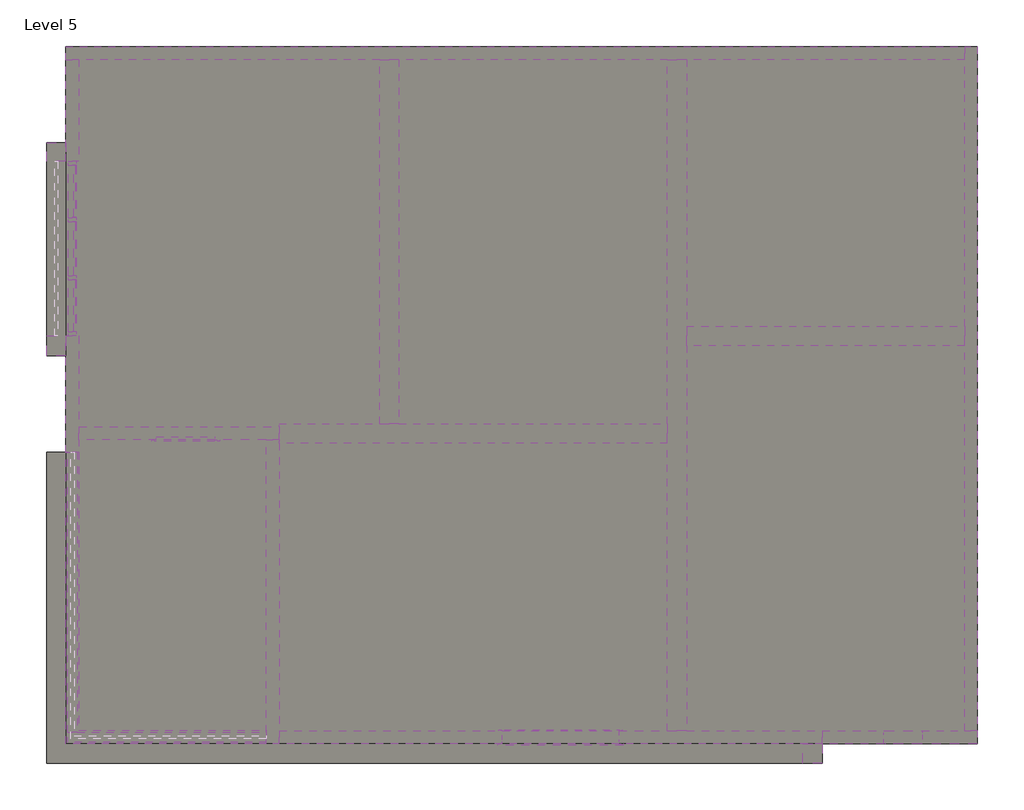
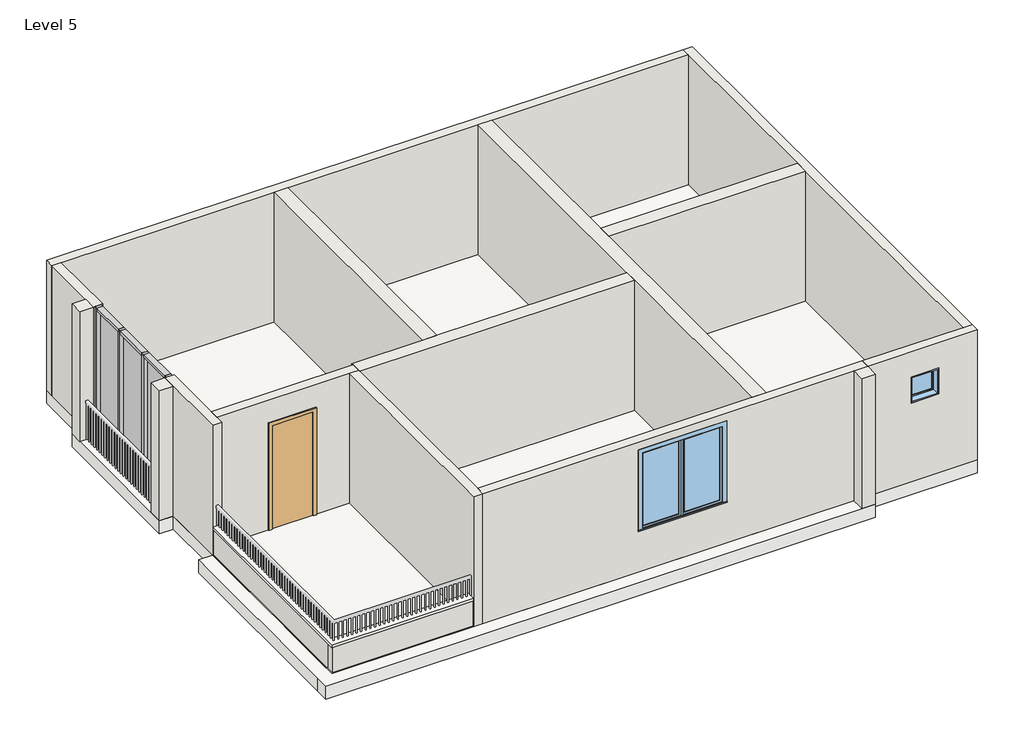
# One storey, part 1 of 2: 17 walls, 10 members, 3 plates, 3 slabs, 2 windows, 1 door.
"""IFC4 building model written with IfcOpenShell, lengths in millimetres."""

from ifc_helpers import new_model, si_unit, frame, origin, place, context, project, spatial, polyline, outline, extrude, faceted_brep, transform, mapped, element, save
from components import door_f936a269, member_eaba9652, member_3f395ae9, member_c17f1be2, member_d2e7e466, system_panel_glazed_52d31088, system_panel_glazed_f0722de2, window_97c6202a, window_6846e476

model = new_model("IFC4")

# Units and contexts
model_context = context("Model", 3, world=origin())
ifc_project = project(units=[si_unit("LENGTHUNIT", "METRE", prefix="MILLI")], contexts=[model_context])

# Site, building, storey
site = spatial("IfcSite", under=ifc_project)
building = spatial("IfcBuilding", under=site)
storey = spatial("IfcBuildingStorey", under=building, Name="Level 5", Elevation=12192.0)

# Door
placement = place(None, origin())
door_shape = door_f936a269(model_context)
element("IfcDoor", 1, ObjectType="Single-Flush : 36\" x 96\"", at=placement, inside=storey, context=model_context, shape_type="MappedRepresentation", body=[
    mapped(door_shape, transform((-16449.2169582, -4610.4617616, 13411.2), x_axis=(-1.0, 0.0, 0.0), y_axis=(0.0, -1.0, 0.0), z_axis=(0.0, 0.0, 1.0))),
])

# Members
member_shape = member_eaba9652(model_context)
element("IfcMember", 2, ObjectType="Rectangular Mullion : 2.5\" x 5\" rectangular", at=placement, inside=storey, context=model_context, shape_type="MappedRepresentation", body=[
    mapped(member_shape, transform((-18227.2169582, -1251.3117616, 13411.2), x_axis=(0.0, -1.0, 0.0), y_axis=(-1.0, 0.0, 0.0), z_axis=(0.0, 0.0, -1.0))),
])
element("IfcMember", 3, ObjectType="Rectangular Mullion : 2.5\" x 5\" rectangular", at=placement, inside=storey, context=model_context, shape_type="MappedRepresentation", body=[
    mapped(member_shape, transform((-18227.2169582, -2165.7117616, 13411.2), x_axis=(0.0, -1.0, 0.0), y_axis=(-1.0, 0.0, 0.0), z_axis=(0.0, 0.0, -1.0))),
])
member_2_shape = member_3f395ae9(model_context)
element("IfcMember", 4, ObjectType="Rectangular Mullion : 2.5\" x 5\" rectangular", at=placement, inside=storey, context=model_context, shape_type="MappedRepresentation", body=[
    mapped(member_2_shape, transform((-18227.2169582, -3080.1117616, 13411.2), x_axis=(0.0, -1.0, 0.0), y_axis=(-1.0, 0.0, 0.0), z_axis=(0.0, 0.0, -1.0))),
])
element("IfcMember", 5, ObjectType="Rectangular Mullion : 2.5\" x 5\" rectangular", at=placement, inside=storey, context=model_context, shape_type="MappedRepresentation", body=[
    mapped(member_2_shape, transform((-18227.2169582, -336.9117616, 16459.2), x_axis=(0.0, 1.0, 0.0), y_axis=(-1.0, 0.0, 0.0), z_axis=(0.0, 0.0, 1.0))),
])
member_3_shape = member_c17f1be2(model_context)
element("IfcMember", 6, ObjectType="Rectangular Mullion : 2.5\" x 5\" rectangular", at=placement, inside=storey, context=model_context, shape_type="MappedRepresentation", body=[
    mapped(member_3_shape, transform((-18227.2169582, -3016.6117616, 16459.2), x_axis=(0.0, 0.0, 1.0), y_axis=(-1.0, 0.0, 0.0), z_axis=(0.0, -1.0, 0.0))),
])
element("IfcMember", 7, ObjectType="Rectangular Mullion : 2.5\" x 5\" rectangular", at=placement, inside=storey, context=model_context, shape_type="MappedRepresentation", body=[
    mapped(member_3_shape, transform((-18227.2169582, -1219.5617616, 16459.2), x_axis=(0.0, 0.0, 1.0), y_axis=(-1.0, 0.0, 0.0), z_axis=(0.0, -1.0, 0.0))),
])
element("IfcMember", 8, ObjectType="Rectangular Mullion : 2.5\" x 5\" rectangular", at=placement, inside=storey, context=model_context, shape_type="MappedRepresentation", body=[
    mapped(member_3_shape, transform((-18227.2169582, -400.4117616, 13411.2), x_axis=(0.0, 0.0, -1.0), y_axis=(-1.0, 0.0, 0.0), z_axis=(0.0, 1.0, 0.0))),
])
element("IfcMember", 9, ObjectType="Rectangular Mullion : 2.5\" x 5\" rectangular", at=placement, inside=storey, context=model_context, shape_type="MappedRepresentation", body=[
    mapped(member_3_shape, transform((-18227.2169582, -2197.4617616, 13411.2), x_axis=(0.0, 0.0, -1.0), y_axis=(-1.0, 0.0, 0.0), z_axis=(0.0, 1.0, 0.0))),
])
member_4_shape = member_d2e7e466(model_context)
element("IfcMember", 10, ObjectType="Rectangular Mullion : 2.5\" x 5\" rectangular", at=placement, inside=storey, context=model_context, shape_type="MappedRepresentation", body=[
    mapped(member_4_shape, transform((-18227.2169582, -1283.0617616, 13411.2), x_axis=(0.0, 0.0, -1.0), y_axis=(-1.0, 0.0, 0.0), z_axis=(0.0, 1.0, 0.0))),
])
element("IfcMember", 11, ObjectType="Rectangular Mullion : 2.5\" x 5\" rectangular", at=placement, inside=storey, context=model_context, shape_type="MappedRepresentation", body=[
    mapped(member_4_shape, transform((-18227.2169582, -2133.9617616, 16459.2), x_axis=(0.0, 0.0, 1.0), y_axis=(-1.0, 0.0, 0.0), z_axis=(0.0, -1.0, 0.0))),
])

# Plates
system_panel_glazed_shape = system_panel_glazed_52d31088(model_context)
element("IfcPlate", 12, ObjectType="System Panel : Glazed", at=placement, inside=storey, context=model_context, shape_type="MappedRepresentation", body=[
    mapped(system_panel_glazed_shape, transform((-18227.2169582, -809.9867616, 13474.7), x_axis=(0.0, -1.0, 0.0), y_axis=(1.0, 0.0, 0.0), z_axis=(0.0, 0.0, 1.0))),
])
element("IfcPlate", 13, ObjectType="System Panel : Glazed", at=placement, inside=storey, context=model_context, shape_type="MappedRepresentation", body=[
    mapped(system_panel_glazed_shape, transform((-18227.2169582, -2607.0367616, 13474.7), x_axis=(0.0, -1.0, 0.0), y_axis=(1.0, 0.0, 0.0), z_axis=(0.0, 0.0, 1.0))),
])
system_panel_glazed_2_shape = system_panel_glazed_f0722de2(model_context)
element("IfcPlate", 14, ObjectType="System Panel : Glazed", at=placement, inside=storey, context=model_context, shape_type="MappedRepresentation", body=[
    mapped(system_panel_glazed_2_shape, transform((-18227.2169582, -1708.5117616, 13474.7), x_axis=(0.0, -1.0, 0.0), y_axis=(1.0, 0.0, 0.0), z_axis=(0.0, 0.0, 1.0))),
])

# Slabs
element("IfcSlab", 15, ObjectType="Generic - 12\"", at=placement, inside=storey, context=model_context, shape_type="SweptSolid", body=[
    extrude(outline(polyline([(-18633.6169582, -41.6299243), (-18328.8169582, -41.6299243), (-18328.8169582, -3394.4299243), (-18633.6169582, -3394.4299243), (-18633.6169582, -41.6299243)])), frame((0.0, 0.0, 13106.4), z_axis=(0.0, 0.0, 1.0), x_axis=(1.0, 0.0, 0.0)), (0.0, 0.0, 1.0), 304.8),
    extrude(outline(polyline([(-18633.6169582, -4908.9117616), (-18328.8169582, -4908.9117616), (-18328.8169582, -9487.2617616), (-6444.7919582, -9487.2617616), (-6444.7919582, -9792.0617616), (-18633.6169582, -9792.0617616), (-18633.6169582, -9487.2617616), (-18633.6169582, -4908.9117616)])), frame((0.0, 0.0, 13106.4), z_axis=(0.0, 0.0, 1.0), x_axis=(1.0, 0.0, 0.0)), (0.0, 0.0, 1.0), 304.8),
])
element("IfcSlab", 16, ObjectType="Generic - 12\" 2", at=placement, inside=storey, context=model_context, shape_type="SweptSolid", body=[
    extrude(outline(polyline([(-4006.3919582, 1466.4882384), (-4006.3919582, -9487.2617616), (-18328.8169582, -9487.2617616), (-18328.8169582, 1466.4882384), (-4006.3919582, 1466.4882384)])), frame((0.0, 0.0, 13106.4), z_axis=(0.0, 0.0, 1.0), x_axis=(1.0, 0.0, 0.0)), (0.0, 0.0, 1.0), 304.8),
])
element("IfcSlab", 17, ObjectType="Generic - 2\"", at=placement, inside=storey, context=model_context, shape_type="SweptSolid", body=[
    extrude(outline(polyline([(-15179.2169582, -9487.2617616), (-18328.8169582, -9487.2617616), (-18328.8169582, -4908.9117616), (-18125.6169582, -4908.9117616), (-18125.6169582, -9277.7117616), (-15179.2169582, -9277.7117616), (-15179.2169582, -9309.4617616), (-15179.2169582, -9487.2617616)])), frame((0.0, 0.0, 14020.8), z_axis=(0.0, 0.0, 1.0), x_axis=(1.0, 0.0, 0.0)), (0.0, 0.0, 1.0), 50.8),
])

# Walls
element("IfcWall", 18, ObjectType="Generic - 12\" white", at=placement, inside=storey, context=model_context, shape_type="SweptSolid", body=[
    extrude(outline(polyline([(-18633.6169582, -336.9117616), (-18633.6169582, -41.6299243), (-18328.8169582, -41.6299243), (-18328.8169582, -336.9117616), (-18633.6169582, -336.9117616)])), frame((0.0, 0.0, 13411.2), z_axis=(0.0, 0.0, 1.0), x_axis=(1.0, 0.0, 0.0)), (0.0, 0.0, 1.0), 3048.0),
])
element("IfcWall", 19, ObjectType="Generic - 12\" white", at=placement, inside=storey, context=model_context, shape_type="SweptSolid", body=[
    extrude(outline(polyline([(-18328.8169582, -3080.1117616), (-18328.8169582, -3394.4299243), (-18633.6169582, -3394.4299243), (-18633.6169582, -3080.1117616), (-18328.8169582, -3080.1117616)])), frame((0.0, 0.0, 13411.2), z_axis=(0.0, 0.0, 1.0), x_axis=(1.0, 0.0, 0.0)), (0.0, 0.0, 1.0), 3048.0),
])
element("IfcWall", 20, ObjectType="Generic - 12\" white", at=placement, inside=storey, context=model_context, shape_type="SweptSolid", body=[
    extrude(outline(polyline([(-6749.5919582, -9487.2617616), (-6444.7919582, -9487.2617616), (-6444.7919582, -9792.0617616), (-6749.5919582, -9792.0617616), (-6749.5919582, -9487.2617616)])), frame((0.0, 0.0, 13411.2), z_axis=(0.0, 0.0, 1.0), x_axis=(1.0, 0.0, 0.0)), (0.0, 0.0, 1.0), 3048.0),
])
element("IfcWall", 21, ObjectType="Generic - 12\" white", at=placement, inside=storey, context=model_context, shape_type="Brep", body=[
    faceted_brep([(-8575.2169582, -9284.0617616, 13411.2), (-8575.2169582, -3232.5117616, 13411.2), (-8575.2169582, -2927.7117616, 13411.2), (-8575.2169582, 1263.2882384, 13411.2), (-8575.2169582, 1263.2882384, 16459.2), (-8575.2169582, -2927.7117616, 16459.2), (-8575.2169582, -3232.5117616, 16459.2), (-8575.2169582, -9284.0617616, 16459.2), (-8880.0169582, -9284.0617616, 13411.2), (-8880.0169582, -9284.0617616, 16459.2), (-8880.0169582, -4762.8617616, 16459.2), (-8880.0169582, -4458.0617616, 16459.2), (-8880.0169582, 1263.2882384, 16459.2), (-8880.0169582, 1263.2882384, 13411.2), (-8880.0169582, -4458.0617616, 13411.2), (-8880.0169582, -4762.8617616, 13411.2)], [[[0, 1, 2, 3, 4, 5, 6, 7]], [[8, 9, 10, 11, 12, 13, 14, 15]], [[3, 2, 1, 0, 8, 15, 14, 13]], [[7, 6, 5, 4, 12, 11, 10, 9]], [[4, 3, 13, 12]], [[0, 7, 9, 8]]]),
])
element("IfcWall", 22, ObjectType="Generic - 12\" white", at=placement, inside=storey, context=model_context, shape_type="Brep", body=[
    faceted_brep([(-14976.0169582, -4762.8617616, 13411.2), (-8880.0169582, -4762.8617616, 13411.2), (-8880.0169582, -4762.8617616, 16459.2), (-14976.0169582, -4762.8617616, 16459.2), (-14976.0169582, -4458.0617616, 13411.2), (-14976.0169582, -4458.0617616, 16459.2), (-13401.2169582, -4458.0617616, 16459.2), (-13096.4169582, -4458.0617616, 16459.2), (-8880.0169582, -4458.0617616, 16459.2), (-8880.0169582, -4458.0617616, 13411.2), (-13096.4169582, -4458.0617616, 13411.2), (-13401.2169582, -4458.0617616, 13411.2), (-14976.0169582, -4712.0617616, 13411.2), (-14976.0169582, -4508.8617616, 13411.2), (-14976.0169582, -4508.8617616, 16459.2), (-14976.0169582, -4712.0617616, 16459.2)], [[[0, 1, 2, 3]], [[4, 5, 6, 7, 8, 9, 10, 11]], [[1, 0, 12, 13, 4, 11, 10, 9]], [[3, 2, 8, 7, 6, 5, 14, 15]], [[0, 3, 15, 14, 5, 4, 13, 12]], [[2, 1, 9, 8]]]),
])
element("IfcWall", 23, ObjectType="Generic - 12\" white", at=placement, inside=storey, context=model_context, shape_type="SweptSolid", body=[
    extrude(outline(polyline([(-13096.4169582, 1263.2882384), (-13096.4169582, -4458.0617616), (-13401.2169582, -4458.0617616), (-13401.2169582, 1263.2882384), (-13096.4169582, 1263.2882384)])), frame((0.0, 0.0, 13411.2), z_axis=(0.0, 0.0, 1.0), x_axis=(1.0, 0.0, 0.0)), (0.0, 0.0, 1.0), 3048.0),
])
element("IfcWall", 24, ObjectType="Generic - 12\" white", at=placement, inside=storey, context=model_context, shape_type="SweptSolid", body=[
    extrude(outline(polyline([(-4209.5919582, -3232.5117616), (-8575.2169582, -3232.5117616), (-8575.2169582, -2927.7117616), (-4209.5919582, -2927.7117616), (-4209.5919582, -3232.5117616)])), frame((0.0, 0.0, 13411.2), z_axis=(0.0, 0.0, 1.0), x_axis=(1.0, 0.0, 0.0)), (0.0, 0.0, 1.0), 3048.0),
])
element("IfcWall", 25, ObjectType="Generic - 6\"", at=placement, inside=storey, context=model_context, shape_type="Brep", body=[
    faceted_brep([(-15179.2169582, -9309.4617616, 13411.2), (-18151.0169582, -9309.4617616, 13411.2), (-18303.4169582, -9309.4617616, 13411.2), (-18303.4169582, -9309.4617616, 14020.8), (-18151.0169582, -9309.4617616, 14020.8), (-15179.2169582, -9309.4617616, 14020.8), (-15179.2169582, -9461.8617616, 13411.2), (-15179.2169582, -9461.8617616, 14020.8), (-18303.4169582, -9461.8617616, 14020.8), (-18303.4169582, -9461.8617616, 13411.2)], [[[0, 1, 2, 3, 4, 5]], [[6, 7, 8, 9]], [[2, 1, 0, 6, 9]], [[5, 4, 3, 8, 7]], [[0, 5, 7, 6]], [[3, 2, 9, 8]]]),
])
element("IfcWall", 26, ObjectType="Generic - 6\"", at=placement, inside=storey, context=model_context, shape_type="SweptSolid", body=[
    extrude(outline(polyline([(-18151.0169582, -4908.9117616), (-18151.0169582, -9309.4617616), (-18303.4169582, -9309.4617616), (-18303.4169582, -4908.9117616), (-18151.0169582, -4908.9117616)])), frame((0.0, 0.0, 13411.2), z_axis=(0.0, 0.0, 1.0), x_axis=(1.0, 0.0, 0.0)), (0.0, 0.0, 1.0), 609.6),
])
element("IfcWall", 27, ObjectType="Generic - 8\"", at=placement, inside=storey, context=model_context, shape_type="Brep", body=[
    faceted_brep([(-4006.3919582, -9284.0617616, 13411.2), (-4006.3919582, 1466.4882384, 13411.2), (-4006.3919582, 1466.4882384, 16459.2), (-4006.3919582, -9284.0617616, 16459.2), (-4209.5919582, -9284.0617616, 13411.2), (-4209.5919582, -9284.0617616, 16459.2), (-4209.5919582, -3232.5117616, 16459.2), (-4209.5919582, -2927.7117616, 16459.2), (-4209.5919582, 1263.2882384, 16459.2), (-4209.5919582, 1466.4882384, 16459.2), (-4209.5919582, 1466.4882384, 13411.2), (-4209.5919582, 1263.2882384, 13411.2), (-4209.5919582, -2927.7117616, 13411.2), (-4209.5919582, -3232.5117616, 13411.2)], [[[0, 1, 2, 3]], [[4, 5, 6, 7, 8, 9, 10, 11, 12, 13]], [[1, 0, 4, 13, 12, 11, 10]], [[3, 2, 9, 8, 7, 6, 5]], [[0, 3, 5, 4]], [[2, 1, 10, 9]]]),
])
element("IfcWall", 28, ObjectType="Generic - 8\"", at=placement, inside=storey, context=model_context, shape_type="Brep", body=[
    faceted_brep([(-4209.5919582, 1466.4882384, 13411.2), (-18328.8169582, 1466.4882384, 13411.2), (-18328.8169582, 1466.4882384, 16459.2), (-4209.5919582, 1466.4882384, 16459.2), (-4209.5919582, 1263.2882384, 13411.2), (-4209.5919582, 1263.2882384, 16459.2), (-8575.2169582, 1263.2882384, 16459.2), (-8880.0169582, 1263.2882384, 16459.2), (-13096.4169582, 1263.2882384, 16459.2), (-13401.2169582, 1263.2882384, 16459.2), (-18125.6169582, 1263.2882384, 16459.2), (-18328.8169582, 1263.2882384, 16459.2), (-18328.8169582, 1263.2882384, 13411.2), (-18125.6169582, 1263.2882384, 13411.2), (-13401.2169582, 1263.2882384, 13411.2), (-13096.4169582, 1263.2882384, 13411.2), (-8880.0169582, 1263.2882384, 13411.2), (-8575.2169582, 1263.2882384, 13411.2)], [[[0, 1, 2, 3]], [[4, 5, 6, 7, 8, 9, 10, 11, 12, 13, 14, 15, 16, 17]], [[1, 0, 4, 17, 16, 15, 14, 13, 12]], [[3, 2, 11, 10, 9, 8, 7, 6, 5]], [[0, 3, 5, 4]], [[2, 1, 12, 11]]]),
])
element("IfcWall", 29, ObjectType="Generic - 8\"", at=placement, inside=storey, context=model_context, shape_type="SweptSolid", body=[
    extrude(outline(polyline([(-18328.8169582, -336.9117616), (-18328.8169582, 1263.2882384), (-18125.6169582, 1263.2882384), (-18125.6169582, -336.9117616), (-18328.8169582, -336.9117616)])), frame((0.0, 0.0, 13411.2), z_axis=(0.0, 0.0, 1.0), x_axis=(1.0, 0.0, 0.0)), (0.0, 0.0, 1.0), 3048.0),
])
element("IfcWall", 30, ObjectType="Generic - 8\"", at=placement, inside=storey, context=model_context, shape_type="Brep", body=[
    faceted_brep([(-18328.8169582, -3080.1117616, 13411.2), (-18328.8169582, -4908.9117616, 13411.2), (-18328.8169582, -4908.9117616, 16459.2), (-18328.8169582, -3080.1117616, 16459.2), (-18125.6169582, -3080.1117616, 13411.2), (-18125.6169582, -3080.1117616, 16459.2), (-18125.6169582, -4508.8617616, 16459.2), (-18125.6169582, -4712.0617616, 16459.2), (-18125.6169582, -4908.9117616, 16459.2), (-18125.6169582, -4908.9117616, 13411.2), (-18125.6169582, -4712.0617616, 13411.2), (-18125.6169582, -4508.8617616, 13411.2), (-18151.0169582, -4908.9117616, 13411.2), (-18303.4169582, -4908.9117616, 13411.2)], [[[0, 1, 2, 3]], [[4, 5, 6, 7, 8, 9, 10, 11]], [[1, 0, 4, 11, 10, 9, 12, 13]], [[2, 1, 13, 12, 9, 8]], [[3, 2, 8, 7, 6, 5]], [[0, 3, 5, 4]]]),
])
element("IfcWall", 31, ObjectType="Generic - 8\" 2", at=placement, inside=storey, context=model_context, shape_type="Brep", body=[
    faceted_brep([(-4006.3919582, -9284.0617616, 13411.2), (-4209.5919582, -9284.0617616, 13411.2), (-6444.7919582, -9284.0617616, 13411.2), (-6444.7919582, -9284.0617616, 16459.2), (-4209.5919582, -9284.0617616, 16459.2), (-4006.3919582, -9284.0617616, 16459.2), (-4869.9919582, -9284.0617616, 15867.4087386), (-5479.5919582, -9284.0617616, 15867.4087386), (-5479.5919582, -9284.0617616, 15257.8087386), (-4869.9919582, -9284.0617616, 15257.8087386), (-4006.3919582, -9487.2617616, 13411.2), (-4006.3919582, -9487.2617616, 16459.2), (-6444.7919582, -9487.2617616, 16459.2), (-6444.7919582, -9487.2617616, 13411.2), (-4869.9919582, -9487.2617616, 15867.4087386), (-4869.9919582, -9487.2617616, 15257.8087386), (-5479.5919582, -9487.2617616, 15257.8087386), (-5479.5919582, -9487.2617616, 15867.4087386)], [[[0, 1, 2, 3, 4, 5], [6, 7, 8, 9]], [[10, 11, 12, 13], [14, 15, 16, 17]], [[2, 1, 0, 10, 13]], [[3, 2, 13, 12]], [[5, 4, 3, 12, 11]], [[0, 5, 11, 10]], [[15, 14, 6, 9]], [[16, 15, 9, 8]], [[17, 16, 8, 7]], [[14, 17, 7, 6]]]),
])
element("IfcWall", 32, ObjectType="Generic - 8\" 3", at=placement, inside=storey, context=model_context, shape_type="Brep", body=[
    faceted_brep([(-14976.0169582, -4712.0617616, 16459.2), (-15179.2169582, -4712.0617616, 16459.2), (-18125.6169582, -4712.0617616, 16459.2), (-18125.6169582, -4712.0617616, 13411.2), (-16906.4169582, -4712.0617616, 13411.2), (-16906.4169582, -4712.0617616, 15849.6), (-15992.0169582, -4712.0617616, 15849.6), (-15992.0169582, -4712.0617616, 13411.2), (-15179.2169582, -4712.0617616, 13411.2), (-14976.0169582, -4712.0617616, 13411.2), (-18125.6169582, -4508.8617616, 16459.2), (-14976.0169582, -4508.8617616, 16459.2), (-14976.0169582, -4508.8617616, 13411.2), (-15992.0169582, -4508.8617616, 13411.2), (-15992.0169582, -4508.8617616, 15849.6), (-16906.4169582, -4508.8617616, 15849.6), (-16906.4169582, -4508.8617616, 13411.2), (-18125.6169582, -4508.8617616, 13411.2)], [[[0, 1, 2, 3, 4, 5, 6, 7, 8, 9]], [[10, 11, 12, 13, 14, 15, 16, 17]], [[3, 17, 16, 4]], [[12, 9, 8, 7, 13]], [[2, 1, 0, 11, 10]], [[3, 2, 10, 17]], [[0, 9, 12, 11]], [[15, 5, 4, 16]], [[5, 15, 14, 6]], [[6, 14, 13, 7]]]),
])
element("IfcWall", 33, ObjectType="Generic - 8\" 3", at=placement, inside=storey, context=model_context, shape_type="Brep", body=[
    faceted_brep([(-15179.2169582, -4712.0617616, 13411.2), (-15179.2169582, -9309.4617616, 13411.2), (-15179.2169582, -9461.8617616, 13411.2), (-15179.2169582, -9487.2617616, 13411.2), (-15179.2169582, -9487.2617616, 16459.2), (-15179.2169582, -4712.0617616, 16459.2), (-14976.0169582, -4712.0617616, 13411.2), (-14976.0169582, -4712.0617616, 16459.2), (-14976.0169582, -4762.8617616, 16459.2), (-14976.0169582, -9284.0617616, 16459.2), (-14976.0169582, -9487.2617616, 16459.2), (-14976.0169582, -9487.2617616, 13411.2), (-14976.0169582, -9284.0617616, 13411.2), (-14976.0169582, -4762.8617616, 13411.2)], [[[0, 1, 2, 3, 4, 5]], [[6, 7, 8, 9, 10, 11, 12, 13]], [[3, 2, 1, 0, 6, 13, 12, 11]], [[5, 4, 10, 9, 8, 7]], [[0, 5, 7, 6]], [[3, 11, 10, 4]]]),
])
element("IfcWall", 34, ObjectType="Generic - 8\" 3", at=placement, inside=storey, context=model_context, shape_type="Brep", body=[
    faceted_brep([(-6444.7919582, -9284.0617616, 13411.2), (-8575.2169582, -9284.0617616, 13411.2), (-8880.0169582, -9284.0617616, 13411.2), (-14976.0169582, -9284.0617616, 13411.2), (-14976.0169582, -9284.0617616, 16459.2), (-8880.0169582, -9284.0617616, 16459.2), (-8575.2169582, -9284.0617616, 16459.2), (-6444.7919582, -9284.0617616, 16459.2), (-11470.8169582, -9284.0617616, 16209.4375963), (-11470.8169582, -9284.0617616, 14380.6375963), (-9642.0169582, -9284.0617616, 14380.6375963), (-9642.0169582, -9284.0617616, 16209.4375963), (-6444.7919582, -9487.2617616, 13411.2), (-6444.7919582, -9487.2617616, 16459.2), (-14976.0169582, -9487.2617616, 16459.2), (-14976.0169582, -9487.2617616, 13411.2), (-11470.8169582, -9487.2617616, 16209.4375963), (-9642.0169582, -9487.2617616, 16209.4375963), (-9642.0169582, -9487.2617616, 14380.6375963), (-11470.8169582, -9487.2617616, 14380.6375963)], [[[0, 1, 2, 3, 4, 5, 6, 7], [8, 9, 10, 11]], [[12, 13, 14, 15], [16, 17, 18, 19]], [[3, 2, 1, 0, 12, 15]], [[7, 6, 5, 4, 14, 13]], [[0, 7, 13, 12]], [[3, 15, 14, 4]], [[9, 8, 16, 19]], [[10, 9, 19, 18]], [[11, 10, 18, 17]], [[8, 11, 17, 16]]]),
])

# Windows
window_shape = window_97c6202a(model_context)
element("IfcWindow", 35, ObjectType="Casement Dbl with Trim.0001 : 72\" x 72\"", at=placement, inside=storey, context=model_context, shape_type="MappedRepresentation", body=[
    mapped(window_shape, transform((-10556.4169582, -9366.6117616, 13466.2375963), x_axis=(-1.0, 0.0, 0.0), y_axis=(0.0, -1.0, 0.0), z_axis=(0.0, 0.0, 1.0))),
])
window_2_shape = window_6846e476(model_context)
element("IfcWindow", 36, ObjectType="Fixed : 24\" x 24\"", at=placement, inside=storey, context=model_context, shape_type="MappedRepresentation", body=[
    mapped(window_2_shape, transform((-5136.6919582, -9385.6617616, 14343.4087386), x_axis=(1.0, 0.0, 0.0), y_axis=(0.0, 1.0, 0.0), z_axis=(0.0, 0.0, 1.0))),
])

save(model, "model.ifc")

# Revit data of these elements
# Type "Single-Flush : 36\" x 96\""
#   Type Mark = "1"
#   Construction Type Id = "MDOOR"
#   Assembly Code = "C1020"
#   Analytic Construction = "Metal"
#   Thickness = 0' - 2"
#   Heat Transfer Coefficient (U) = 0.651978 BTU/(h·ft²·°F)
#   Height = 8' - 0"
#   Trim Projection Ext = 0' - 1"
#   Trim Projection Int = 0' - 1"
#   Trim Width = 0' - 3"
#   Width = 3' - 0"
#   Define Thermal Properties by = 1
#   Door Material = Glass, Clear Glazing
#   Frame Material = Iron, Ductile
#   Visual Light Transmittance = 0
#   Solar Heat Gain Coefficient = 0
#   Function = (empty or 0)
#   Wall Closure = (empty or 0)
# Type "Rectangular Mullion : 2.5\" x 5\" rectangular"
#   built-in parameter 1007304 = 0.416667 (stored number, unit not read)
#   built-in parameter 1007301 = 0.104167 (stored number, unit not read)
#   built-in parameter 1007300 = 0.104167 (stored number, unit not read)
# Type "System Panel : Glazed"
#   Construction Type Id = "GSP4R"
#   Analytic Construction = "1/8 in Pilkington single glazing"
#   Visual Light Transmittance = 0.9
#   Solar Heat Gain Coefficient = 0.86
#   Heat Transfer Coefficient (U) = 1.18115 BTU/(h·ft²·°F)
# Type "Generic - 12\""
#   Assembly Code = "B1010"
#   Function = 0
#   Layers, outside or top first: 1' - 0" "Parking Stripe" (function 1)
# Type "Generic - 12\" 2"
#   Assembly Code = "B1010"
#   Function = 0
#   Layers, outside or top first: 1' - 0" "Parking Stripe" (function 1)
# Type "Generic - 2\""
#   Assembly Code = "B1010"
#   Function = 0
#   Layers, outside or top first: 0' - 2" "Parking Stripe" (function 1)
# Type "Generic - 12\" white"
#   Assembly Code = "B2010"
#   Layers, outside or top first: 1' - 0" "Parking Stripe" (function 1)
# Type "Generic - 6\""
#   Assembly Code = "B2010"
#   Layers, outside or top first: 0' - 6" "Concrete Masonry Units" (function 1)
# Type "Generic - 8\""
#   Assembly Code = "B2010"
#   Layers, outside or top first: 0' - 8" "Door - Frame" (function 1)
# Type "Generic - 8\" 2"
#   Assembly Code = "B2010"
#   Layers, outside or top first: 0' - 8" "Door - Frame" (function 1)
# Type "Generic - 8\" 3"
#   Assembly Code = "B2010"
#   Layers, outside or top first: 0' - 8" "EIFS, Exterior Insulation" (function 1)
# Type "Casement Dbl with Trim.0001 : 72\" x 72\""
#   Type Mark = "10"
#   Construction Type Id = "GSP4R"
#   Assembly Code = "B2020100"
#   Analytic Construction = "1/8 in Pilkington single glazing"
#   Visual Light Transmittance = 0.9
#   Solar Heat Gain Coefficient = 0.78
#   Heat Transfer Coefficient (U) = 0.6496 BTU/(h·ft²·°F)
#   Height = 6' - 0"
#   Default Sill Height = 3' - 0"
#   Trim Projection - Ext. = 0' - 0 1/2"
#   Trim Projection - Int. = 0' - 0 3/4"
#   Trim Width - Exterior = 0' - 3 1/2"
#   Trim Width - Interior = 0' - 3 1/2"
#   Width = 6' - 0"
#   Window Inset = 0' - 0 3/4"
#   Define Thermal Properties by = 1
#   Glass Pane Material = Glass
#   Sash Material = Iron, Ductile
#   Trim Exterior Material = Iron, Ductile
#   Trim Interior Material = Iron, Ductile
#   Wall Closure = (empty or 0)
# Type "Fixed : 24\" x 24\""
#   Type Mark = "3"
#   Construction Type Id = "GSP4R"
#   Assembly Code = "B2020100"
#   Analytic Construction = "1/8 in Pilkington single glazing"
#   Visual Light Transmittance = 0.9
#   Solar Heat Gain Coefficient = 0.78
#   Heat Transfer Coefficient (U) = 0.6496 BTU/(h·ft²·°F)
#   Height = 2' - 0"
#   Default Sill Height = 3' - 0"
#   Width = 2' - 0"
#   Window Inset = 0' - 0 3/4"
#   Define Thermal Properties by = 1
#   Glass Pane Material = Glass
#   Sash Material = Iron, Ductile
#   Wall Closure = (empty or 0)
# Element 1 (IfcDoor, "Single-Flush : 36\" x 96\"")
#   Phase Created = New Construction
#   Materials on its faces: "Iron, Ductile", "Glass, Clear Glazing"
# Elements 2, 3, 4, 5, 6, 7, 8, 9, 10, 11 (IfcMember, "Rectangular Mullion : 2.5\" x 5\" rectangular")
#   Phase Created = New Construction
#   Materials on its faces: "Iron, Ductile"
# Elements 12, 13, 14 (IfcPlate, "System Panel : Glazed")
#   Phase Created = New Construction
#   Materials on its faces: "Glass"
# Element 15 (IfcSlab, "Generic - 12\"")
#   built-in parameter 1001955 = 3.14159 (stored number, unit not read)
#   Height Offset From Level = 4' - 0"
#   Phase Created = New Construction
#   Materials on its faces: "Parking Stripe"
# Element 16 (IfcSlab, "Generic - 12\" 2")
#   Height Offset From Level = 4' - 0"
#   Phase Created = New Construction
#   Materials on its faces: "Parking Stripe"
# Element 17 (IfcSlab, "Generic - 2\"")
#   built-in parameter 1001955 = -1.5708 (stored number, unit not read)
#   Height Offset From Level = 6' - 2"
#   Phase Created = New Construction
#   Materials on its faces: "Parking Stripe"
# Elements 18, 19, 20, 21, 22, 23, 24 (IfcWall, "Generic - 12\" white")
#   built-in parameter 1001111 = 4' - 0"
#   Top Offset = 0' - 0"
#   Base Offset = 4' - 0"
#   Unconnected Height = 10' - 0"
#   wall height = 10' - 0"
#   Phase Created = New Construction
#   Base Constraint = Level 5
#   Materials on its faces: "Parking Stripe"
# Elements 25, 26 (IfcWall, "Generic - 6\"")
#   built-in parameter 1001111 = 4' - 0"
#   Top Offset = 0' - 0"
#   Base Offset = 4' - 0"
#   Unconnected Height = 2' - 0"
#   wall height = 2' - 0"
#   Phase Created = New Construction
#   Base Constraint = Level 5
#   Materials on its faces: "Concrete Masonry Units"
# Elements 27, 28, 29, 30 (IfcWall, "Generic - 8\"")
#   built-in parameter 1001111 = 4' - 0"
#   Top Offset = 0' - 0"
#   Base Offset = 4' - 0"
#   Unconnected Height = 10' - 0"
#   wall height = 10' - 0"
#   Phase Created = New Construction
#   Base Constraint = Level 5
#   Materials on its faces: "Door - Frame"
# Element 31 (IfcWall, "Generic - 8\" 2")
#   built-in parameter 1001111 = 4' - 0"
#   Top Offset = 0' - 0"
#   Base Offset = 4' - 0"
#   Unconnected Height = 10' - 0"
#   wall height = 10' - 0"
#   Phase Created = New Construction
#   Base Constraint = Level 5
#   Materials on its faces: "Door - Frame"
# Elements 32, 33, 34 (IfcWall, "Generic - 8\" 3")
#   built-in parameter 1001111 = 4' - 0"
#   Top Offset = 0' - 0"
#   Base Offset = 4' - 0"
#   Unconnected Height = 10' - 0"
#   wall height = 10' - 0"
#   Phase Created = New Construction
#   Base Constraint = Level 5
#   Materials on its faces: "EIFS, Exterior Insulation"
# Element 35 (IfcWindow, "Casement Dbl with Trim.0001 : 72\" x 72\"")
#   Mark = "8"
#   Phase Created = New Construction
#   Materials on its faces: "Iron, Ductile", "Glass"
# Element 36 (IfcWindow, "Fixed : 24\" x 24\"")
#   Mark = "7"
#   Phase Created = New Construction
#   Materials on its faces: "Iron, Ductile", "Glass"
# Materials
#   "Glass, Clear Glazing": class "Glass", colour RGB 0 128 192, transparency 0.75, Description = "Clear glazing", Cost = 0
#   "Iron, Ductile": class "Metal", colour RGB 0 0 0, transparency 0, Description = "Ductile cast iron", Cost = 0
#   "Parking Stripe": class "Paint", colour RGB 250 250 91, transparency 0, Cost = 0
#   "Concrete Masonry Units": class "Masonry", colour RGB 227 227 227, transparency 0, Description = "Concrete masonry units", Cost = 0
#   "Door - Frame": colour RGB 118 70 51, transparency 0, Cost = 0
#   "EIFS, Exterior Insulation": class "Generic", colour RGB 127 127 127, transparency 0, Description = "EIFS - Exterior Insulation", Cost = 0
#   "Glass": class "Glass", colour RGB 0 128 192, transparency 0.75, Description = "Soda Lime Glass", Cost = 0
